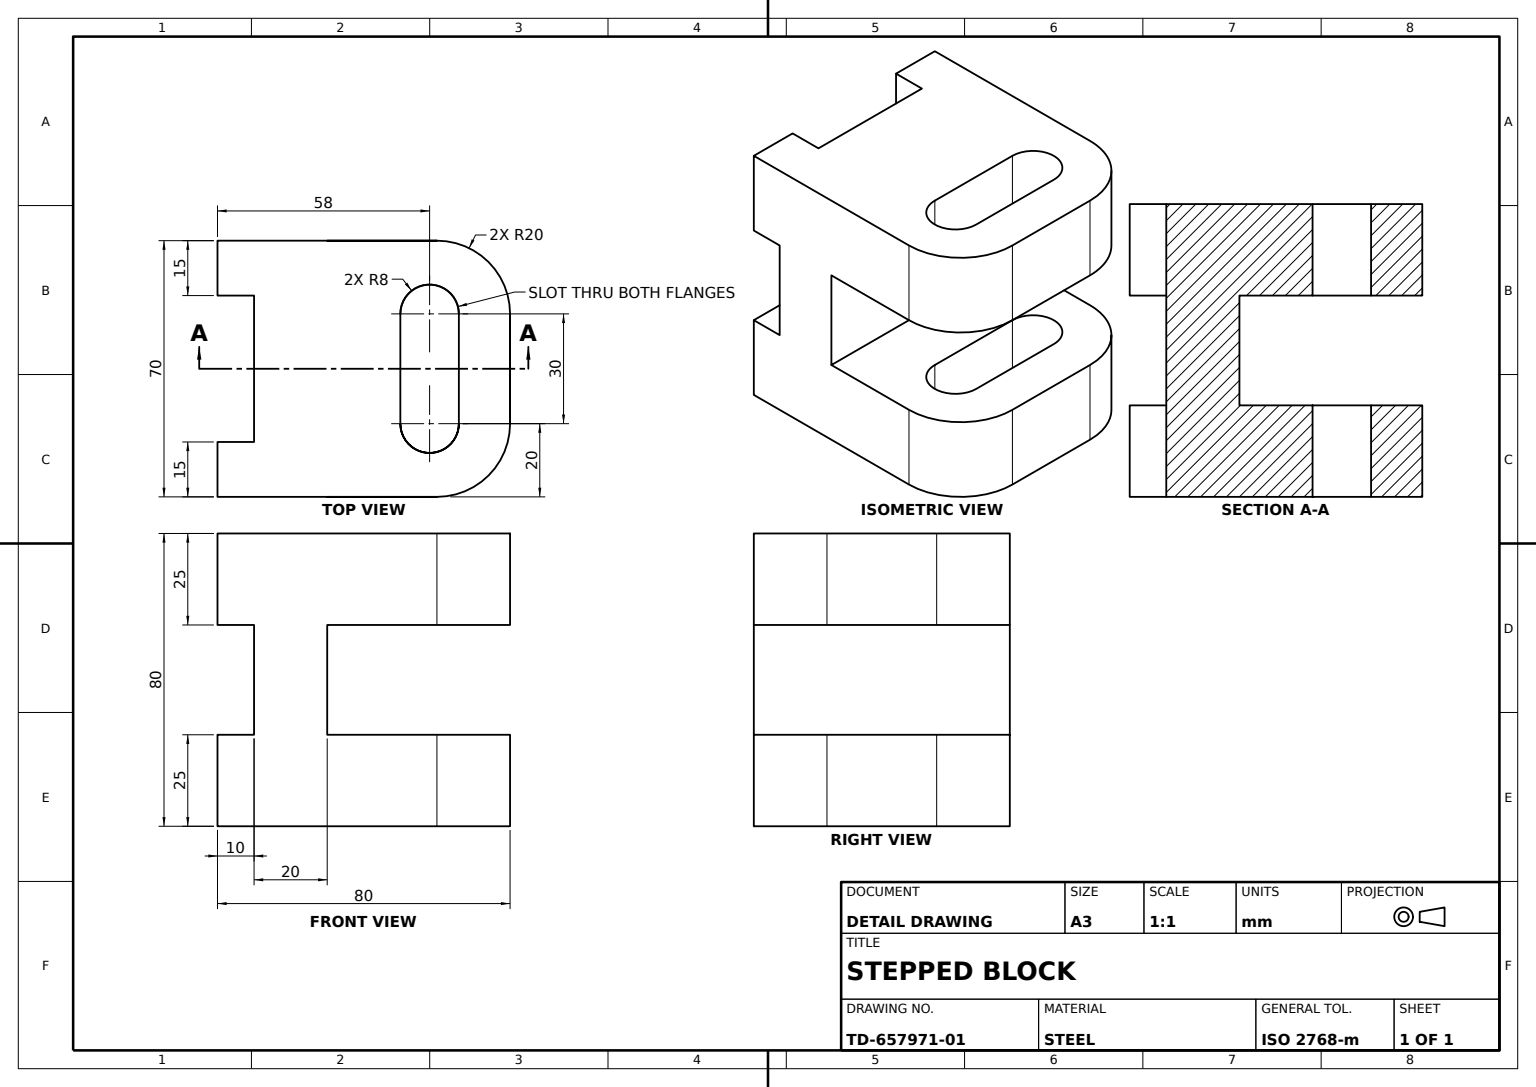
from build123d import *

# Parameters (mm, degrees)
BASE_BLOCK_PROFILE_W           = 70
BASE_BLOCK_PROFILE_H           = 80
BASE_BLOCK_20MM_DEPTH          = 20
H_BOSS_PROFILE_W               = 15
H_BOSS_PROFILE_H               = 25
H_BOSS_10MM_DEPTH              = 10
REAR_BOSS_PROFILE_W            = 70
REAR_BOSS_PROFILE_H            = 50
REAR_BOSS_25MM_DEPTH           = 25
REAR_BOSS_EXTENSION_PROFILE_W  = 70
REAR_BOSS_EXTENSION_PROFILE_H  = 50
REAR_BOSS_EXTENSION_25MM_DEPTH = 25
THROUGH_SLOT_8X30_DEPTH        = 100
LOWER_NOTCH_CUT_DEPTH          = 100


with BuildPart() as part:
    # Base Block Profile → Base Block 20mm (new body)
    with BuildSketch(Plane.XY):
        with Locations((35, 40)):
            Rectangle(BASE_BLOCK_PROFILE_W, BASE_BLOCK_PROFILE_H)
    extrude(amount=BASE_BLOCK_20MM_DEPTH)

    # H Boss Profile → H Boss 10mm (add)
    with BuildSketch(Plane.XY.offset(20)):
        with Locations((7.5, 67.5)):
            Rectangle(H_BOSS_PROFILE_W, H_BOSS_PROFILE_H)
        with Locations((62.5, 67.5)):
            Rectangle(H_BOSS_PROFILE_W, H_BOSS_PROFILE_H)
        with Locations((7.5, 12.5)):
            Rectangle(H_BOSS_PROFILE_W, H_BOSS_PROFILE_H)
        with Locations((62.5, 12.5)):
            Rectangle(H_BOSS_PROFILE_W, H_BOSS_PROFILE_H)
    extrude(amount=H_BOSS_10MM_DEPTH)

    # Rear Boss Profile → Rear Boss 25mm (add)
    with BuildSketch(Plane(origin=(0, 80, 0), x_dir=(1, 0, 0), z_dir=(0, 1, 0))):
        with Locations((35, 25)):
            Rectangle(REAR_BOSS_PROFILE_W, REAR_BOSS_PROFILE_H)
    extrude(amount=-REAR_BOSS_25MM_DEPTH)

    # Rear Boss Extension Profile → Rear Boss Extension 25mm (add)
    with BuildSketch(Plane.XZ):
        with Locations((35, -25)):
            Rectangle(REAR_BOSS_EXTENSION_PROFILE_W, REAR_BOSS_EXTENSION_PROFILE_H)
    extrude(amount=-REAR_BOSS_EXTENSION_25MM_DEPTH)

    # Slot 8x30 Profile → Through Slot 8x30 (cut)
    with BuildSketch(Plane.XZ):
        with BuildLine():
            Line((20, -20), (50, -20))
            ThreePointArc((50, -20), (58, -28), (50, -36))
            Line((50, -36), (20, -36))
            ThreePointArc((20, -36), (12, -28), (20, -20))
        make_face()
    extrude(amount=-THROUGH_SLOT_8X30_DEPTH, mode=Mode.SUBTRACT)

    # Lower Notch Profile → Lower Notch Cut (cut)
    with BuildSketch(Plane.XZ):
        with BuildLine():
            Line((0, -50), (0, -30))
            ThreePointArc((0, -30), (5.857864376, -44.142135624), (20, -50))
            Line((20, -50), (0, -50))
        make_face()
        with BuildLine():
            Line((70, -50), (70, -30))
            ThreePointArc((70, -30), (64.142135624, -44.142135624), (50, -50))
            Line((50, -50), (70, -50))
        make_face()
    extrude(amount=-LOWER_NOTCH_CUT_DEPTH, mode=Mode.SUBTRACT)


solid = part.part
